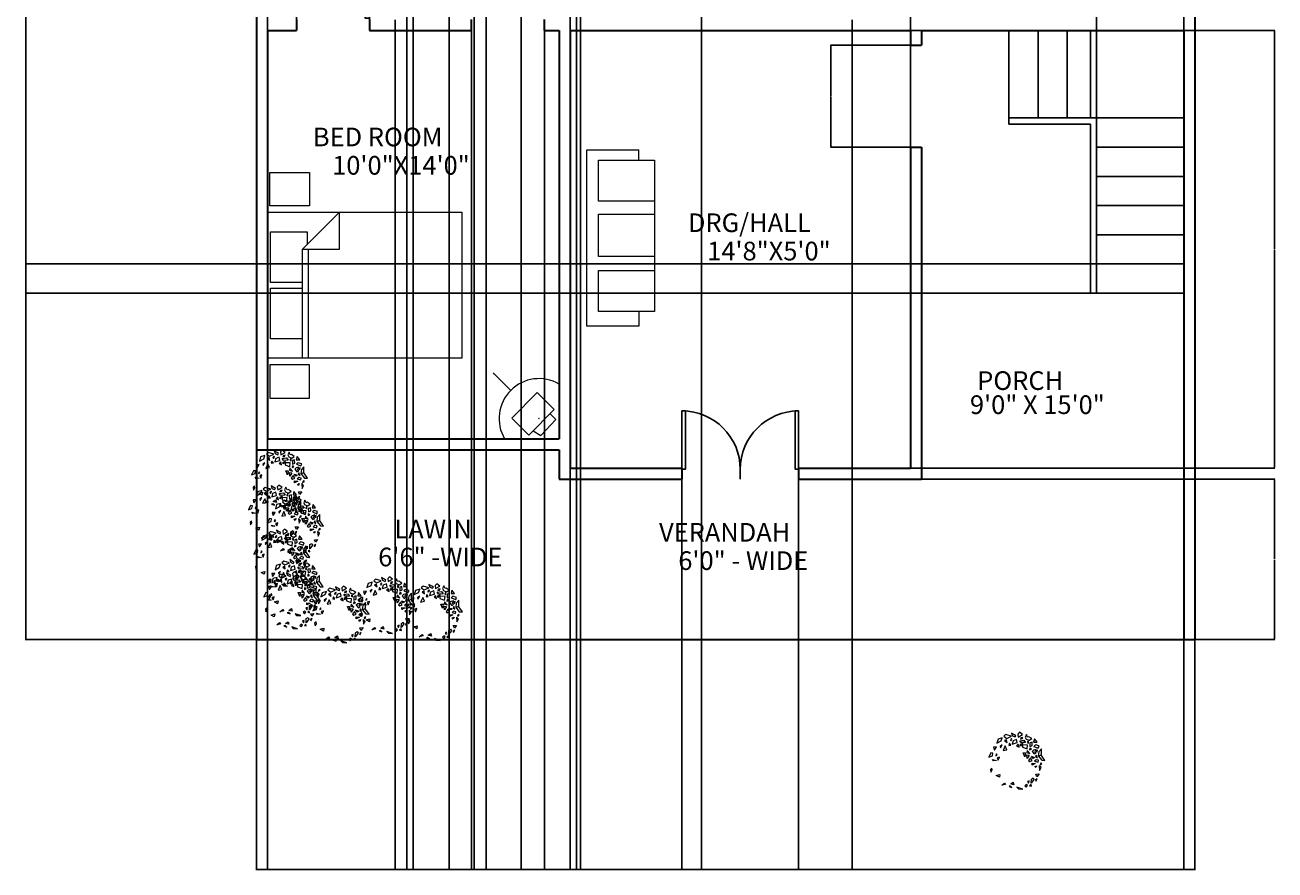
# Model space of a CAD drawing. Units: inches. Extents: x 2337 to 2851, y 1463 to 2183.
# Tile 1 of 4: x 2337 to 2851, y 1463 to 1810. Entities that reach past the tile are written whole.
import ezdxf

# ---------------------------------------------------------------- set-up
doc = ezdxf.new("R2010")
doc.units = ezdxf.units.IN
for name, color, linetype, lineweight in [('A-ANNO-DIMS', 2, 'Continuous', 18), ('A-AREA-IDEN', 7, 'Continuous', 18), ('A-DOOR', 4, 'Continuous', 25), ('A-FLOR-STRS', 7, 'Continuous', 25), ('A-FURN', 8, 'Continuous', 18), ('A-WALL', 7, 'Continuous', 35), ('L-PLNT-TREE', 94, 'Continuous', 13)]:
    doc.layers.add(name, color=color, linetype=linetype, lineweight=lineweight)
doc.styles.get("Standard").update_dxf_attribs({"font": 'arial.ttf'})
doc.dimstyles.get("Standard").update_dxf_attribs({"dimtxt": 0.18, "dimasz": 0.18, "dimexe": 0.18, "dimexo": 0.0625, "dimgap": 0.09, "dimtad": 0, "dimtih": 1, "dimtoh": 1, "dimdec": 4, "dimzin": 0, "dimdsep": 46, "dimtxsty": 'Standard', "dimcen": 0.09, "dimadec": 0, "dimazin": 0, "dimtfac": 1, "dimtdec": 4, "dimtofl": 0, "dimtmove": 0, "dimatfit": 3, "dimfxl": 1, "dimtolj": 1, "dimtzin": 0, "dimarcsym": 0})

# ---------------------------------------------------------------- blocks, each defined once
blk = doc.blocks.new('*U2')
for p, q in [((0, 0), (0, -5)), ((30, 0), (30, -5))]:
    blk.add_line(p, q)
blk.add_lwpolyline([(0, 0), (0, 30), (1.75, 30), (1.75, 0)], close=True)
blk.add_arc((0, 0), 30, 0, 90)
blk = doc.blocks.new('Bed - Queen')
for p, q in [((0, -80.00003), (0, 0)), ((0, 0), (59.99999, 0)), ((59.99999, 0), (59.99999, -80.00003)), ((7.99999, -1.2), (28.79998, -1.2)), ((7.99999, -14.4), (7.99999, -1.2)), ((28.79998, -1.2), (28.79998, -14.4)), ((31.19999, -1.2), (51.99999, -1.2)), ((31.19999, -14.4), (31.19999, -1.2)), ((51.99999, -1.2), (51.99999, -16.4)), ((0, -14.4), (44.8, -14.4)), ((59.99999, -29.6), (44.8, -14.4)), ((44.8, -14.4), (44.8, -29.6)), ((44.8, -16.8), (0, -16.8)), ((51.99999, -16.4), (46.79936, -16.4)), ((44.8, -29.6), (59.99999, -29.6)), ((59.99999, -80.00003), (0, -80.00003))]:
    blk.add_line(p, q)
blk = doc.blocks.new('*U10')
for points in [[(-4.43, 11.05), (-5.18, 10.36), (-3.96, 9.49), (-2.07, 10.36)], [(-2, 11.66), (-1.6, 10.62), (-0.52, 10.1), (-0.18, 10.62), (-0.79, 10.96)], [(1.24, 12), (0.56, 11.31), (0.76, 10.01), (2.52, 11.05)], [(4.14, 11.14), (3.6, 10.01), (4, 9.23), (5.22, 8.71), (6.3, 9.41), (5.08, 10.19), (4.61, 10.01)], [(-8.14, 6.03), (-9.36, 5.95), (-9.02, 4.73)], [(-5.78, 9.75), (-7.54, 9.23), (-8.01, 7.5), (-6.26, 8.45)], [(-5.78, 6.81), (-6.66, 6.21), (-6.52, 5.69)], [(-4.57, 6.38), (-5.45, 4.47), (-3.89, 4.82)], [(-4.84, 8.63), (-3.83, 7.85), (-4.03, 8.97)], [(-2.88, 7.5), (-3.15, 6.64), (-2.27, 6.72)], [(-1.94, 9.49), (-2.48, 8.97), (-2.27, 8.54), (-1.8, 9.06)], [(0.02, 9.06), (-1.33, 8.54), (-1.73, 7.16), (0.29, 7.76)], [(0.76, 7.16), (0.09, 6.46), (1.1, 5.95)], [(1.37, 8.54), (3.13, 8.8), (3.8, 7.85), (1.91, 7.76)], [(2.59, 9.93), (1.84, 9.75), (1.64, 9.23), (2.32, 9.41)], [(1.71, 6.29), (1.71, 7.07), (2.65, 7.5), (2.11, 6.9)], [(2.52, 6.81), (2.52, 5.86), (4.41, 5.17), (4.61, 6.72)], [(4.61, 8.28), (4.54, 7.76), (4.95, 7.59), (4.95, 8.28)], [(5.49, 5.51), (5.42, 4.82), (6.16, 5.08)], [(6.43, 7.94), (5.49, 7.68), (5.56, 6.21), (6.5, 6.64)], [(7.45, 9.32), (7.11, 7.94), (8.52, 7.94)], [(7.85, 6.81), (7.18, 6.21), (9, 5.51), (9.33, 6.38)], [(10.28, 5.17), (9.2, 4.04), (9, 2.31), (10.48, 0.49), (11.76, 0.41), (10.35, 2.48), (9.33, 2.4), (10.28, 2.83)], [(-11.32, 1.79), (-9.83, 2.31), (-9.63, 3.44), (-10.44, 3.52)], [(-8.21, 0.41), (-9.43, 0.32), (-9.83, 0.84)], [(-8.21, 3.09), (-8.48, 2.31), (-7.87, 2.57)], [(-7, 1.79), (-7.94, 1.53), (-7.47, 0.49)], [(3.53, 1.88), (2.86, 3.52), (3.8, 3.52)], [(4.41, 4.56), (4.27, 3.7), (5.49, 3.26)], [(4.27, 2.74), (5.29, 2.66), (4.41, 1.27)], [(5.83, 1.53), (5.02, 0.41), (5.49, -0.02), (6.5, 0.41)], [(7.51, 1.71), (6.91, 1.27), (6.23, 2.14)], [(8.12, 4.99), (7.11, 4.65), (6.5, 4.13), (7.38, 3.09), (8.12, 3.52), (7.65, 3.87)], [(8.12, 0.75), (7.51, 0.15), (8.93, -0.28), (9.13, 0.49)], [(8.19, 2.57), (7.92, 2.05), (8.66, 1.53)], [(8.73, 4.73), (8.19, 4.56), (8.39, 3.87), (8.59, 4.04)], [(-10.03, -2.71), (-10.64, -3.31), (-10.44, -4.44), (-9.9, -3.49)], [(7.78, -0.8), (6.43, -1.5), (6.43, -0.72)], [(8.32, -1.75), (7.98, -2.53), (7.58, -2.1)], [(9.33, -5.13), (8.46, -6.25), (7.98, -5.22)], [(9.33, -1.75), (9.54, -3.74), (10.14, -2.53)], [(10.08, -0.63), (9.74, -1.32), (10.48, -0.89)], [(-8.28, -5.73), (-6.79, -5.3), (-7, -6.51)], [(-4.84, -8.85), (-4.43, -9.45), (-5.99, -9.8)], [(-2.54, -10.06), (-3.02, -10.23), (-1.8, -10.67)], [(-2.34, -9.2), (-1.26, -8.5), (-0.99, -9.54)], [(4.07, -9.45), (3.53, -9.97), (4.07, -10.58), (4.61, -9.89)], [(5.29, -7.98), (4.61, -8.16), (5.02, -8.94)], [(6.03, -9.45), (5.42, -9.97), (6.16, -10.15)], [(6.1, -8.94), (6.16, -7.21), (6.91, -6.69), (7.24, -7.38)], [(8.05, -8.07), (8.59, -7.12), (7.92, -7.55)], [(0.22, -10.58), (0.83, -11.27), (2.59, -11.36)]]:
    blk.add_lwpolyline(points, close=True)
blk = doc.blocks.new('NIGHTSTAND')
blk.add_lwpolyline([(0, 13.73), (16.32, 13.73), (16.32, 0), (0, 0)], close=True)
blk = doc.blocks.new('*D29')
at = {"layer": 'A-ANNO-DIMS', "color": 0, "lineweight": -2, "transparency": 16777216}
for p, q in [((2432.04, 1557.27), (2432.04, 1462.52)), ((2818.04, 1557.27), (2818.04, 1462.52)), ((2432.22, 1462.7), (2624.75, 1462.7)), ((2817.86, 1462.7), (2625.33, 1462.7))]:
    blk.add_line(p, q, dxfattribs=at)
at = {"layer": 'A-ANNO-DIMS', "color": 0, "transparency": 16777216}
for points in [[(2432.22, 1462.73), (2432.22, 1462.67), (2432.04, 1462.7)], [(2817.86, 1462.73), (2817.86, 1462.67), (2818.04, 1462.7)]]:
    blk.add_solid(points, dxfattribs=at)
at = {"layer": 'Defpoints', "color": 0, "transparency": 16777216}
for p in [(2432.04, 1557.33), (2818.04, 1557.33), (2818.04, 1462.7)]:
    blk.add_point(p, dxfattribs=at)
at = {"layer": 'A-ANNO-DIMS', "color": 0, "transparency": 16777216, "insert": (2625.04, 1462.7), "char_height": 0.18, "attachment_point": 5}
blk.add_mtext('\\A1;386', dxfattribs=at)
blk = doc.blocks.new('*D30')
at = {"layer": 'A-ANNO-DIMS', "color": 0, "lineweight": -2, "transparency": 16777216}
for p, q in [((2431.97, 2149.83), (2336.95, 2149.83)), ((2337.13, 2149.65), (2337.13, 1853.76)), ((2337.13, 1557.51), (2337.13, 1853.4)), ((2431.97, 1557.33), (2336.95, 1557.33))]:
    blk.add_line(p, q, dxfattribs=at)
at = {"layer": 'A-ANNO-DIMS', "color": 0, "transparency": 16777216}
for points in [[(2337.1, 2149.65), (2337.16, 2149.65), (2337.13, 2149.83)], [(2337.1, 1557.51), (2337.16, 1557.51), (2337.13, 1557.33)]]:
    blk.add_solid(points, dxfattribs=at)
at = {"layer": 'Defpoints', "color": 0, "transparency": 16777216}
for p in [(2337.13, 2149.83), (2432.04, 2149.83), (2432.04, 1557.33)]:
    blk.add_point(p, dxfattribs=at)
at = {"layer": 'A-ANNO-DIMS', "color": 0, "transparency": 16777216, "insert": (2337.13, 1853.58), "char_height": 0.18, "attachment_point": 5}
blk.add_mtext('\\A1;592.5', dxfattribs=at)
blk = doc.blocks.new('*D32')
at = {"layer": 'A-ANNO-DIMS', "color": 0, "lineweight": -2, "transparency": 16777216}
for p, q in [((2561.04, 1627.89), (2561.04, 2182.75)), ((2561.22, 2182.57), (2630.76, 2182.57)), ((2700.86, 2182.57), (2631.32, 2182.57)), ((2701.04, 1627.89), (2701.04, 2182.75))]:
    blk.add_line(p, q, dxfattribs=at)
at = {"layer": 'A-ANNO-DIMS', "color": 0, "transparency": 16777216}
for points in [[(2561.22, 2182.6), (2561.22, 2182.54), (2561.04, 2182.57)], [(2700.86, 2182.6), (2700.86, 2182.54), (2701.04, 2182.57)]]:
    blk.add_solid(points, dxfattribs=at)
at = {"layer": 'Defpoints', "color": 0, "transparency": 16777216}
for p in [(2701.04, 2182.57), (2561.04, 1627.83), (2701.04, 1627.83)]:
    blk.add_point(p, dxfattribs=at)
at = {"layer": 'A-ANNO-DIMS', "color": 0, "transparency": 16777216, "insert": (2631.04, 2182.57), "char_height": 0.18, "attachment_point": 5}
blk.add_mtext('\\A1;140', dxfattribs=at)
blk = doc.blocks.new('*D33')
at = {"layer": 'A-ANNO-DIMS', "color": 0, "lineweight": -2, "transparency": 16777216}
for p, q in [((2701.1, 1807.83), (2850.96, 1807.83)), ((2850.78, 1807.65), (2850.78, 1718.01)), ((2850.78, 1628.01), (2850.78, 1717.65)), ((2701.1, 1627.83), (2850.96, 1627.83))]:
    blk.add_line(p, q, dxfattribs=at)
at = {"layer": 'A-ANNO-DIMS', "color": 0, "transparency": 16777216}
for points in [[(2850.75, 1807.65), (2850.81, 1807.65), (2850.78, 1807.83)], [(2850.75, 1628.01), (2850.81, 1628.01), (2850.78, 1627.83)]]:
    blk.add_solid(points, dxfattribs=at)
at = {"layer": 'Defpoints', "color": 0, "transparency": 16777216}
for p in [(2701.04, 1807.83), (2850.78, 1807.83), (2701.04, 1627.83)]:
    blk.add_point(p, dxfattribs=at)
at = {"layer": 'A-ANNO-DIMS', "color": 0, "transparency": 16777216, "insert": (2850.78, 1717.83), "char_height": 0.18, "attachment_point": 5}
blk.add_mtext('\\A1;180', dxfattribs=at)
blk = doc.blocks.new('*D35')
at = {"layer": 'A-ANNO-DIMS', "color": 0, "lineweight": -2, "transparency": 16777216}
for p, q in [((2489.04, 1812.27), (2489.04, 1462.52)), ((2677.04, 1812.27), (2677.04, 1462.52)), ((2489.22, 1462.7), (2582.76, 1462.7)), ((2676.86, 1462.7), (2583.32, 1462.7))]:
    blk.add_line(p, q, dxfattribs=at)
at = {"layer": 'A-ANNO-DIMS', "color": 0, "transparency": 16777216}
for points in [[(2489.22, 1462.73), (2489.22, 1462.67), (2489.04, 1462.7)], [(2676.86, 1462.73), (2676.86, 1462.67), (2677.04, 1462.7)]]:
    blk.add_solid(points, dxfattribs=at)
at = {"layer": 'Defpoints', "color": 0, "transparency": 16777216}
for p in [(2489.04, 1812.33), (2677.04, 1812.33), (2677.04, 1462.7)]:
    blk.add_point(p, dxfattribs=at)
at = {"layer": 'A-ANNO-DIMS', "color": 0, "transparency": 16777216, "insert": (2583.04, 1462.7), "char_height": 0.18, "attachment_point": 5}
blk.add_mtext('\\A1;188', dxfattribs=at)
blk = doc.blocks.new('*D37')
at = {"layer": 'A-ANNO-DIMS', "color": 0, "lineweight": -2, "transparency": 16777216}
for p, q in [((2615.04, 2080.77), (2615.04, 1462.52)), ((2813.54, 2080.77), (2813.54, 1462.52)), ((2615.22, 1462.7), (2713.9, 1462.7)), ((2813.36, 1462.7), (2714.67, 1462.7))]:
    blk.add_line(p, q, dxfattribs=at)
at = {"layer": 'A-ANNO-DIMS', "color": 0, "transparency": 16777216}
for points in [[(2615.22, 1462.73), (2615.22, 1462.67), (2615.04, 1462.7)], [(2813.36, 1462.73), (2813.36, 1462.67), (2813.54, 1462.7)]]:
    blk.add_solid(points, dxfattribs=at)
at = {"layer": 'Defpoints', "color": 0, "transparency": 16777216}
for p in [(2615.04, 2080.83), (2813.54, 2080.83), (2813.54, 1462.7)]:
    blk.add_point(p, dxfattribs=at)
at = {"layer": 'A-ANNO-DIMS', "color": 0, "transparency": 16777216, "insert": (2714.29, 1462.7), "char_height": 0.18, "attachment_point": 5}
blk.add_mtext('\\A1;198.5', dxfattribs=at)
blk = doc.blocks.new('*D38')
at = {"layer": 'A-ANNO-DIMS', "color": 0, "lineweight": -2, "transparency": 16777216}
for p, q in [((2496.54, 2080.77), (2496.54, 1462.52)), ((2526.54, 2080.77), (2526.54, 1462.52)), ((2496.72, 1462.7), (2511.32, 1462.7)), ((2526.36, 1462.7), (2511.76, 1462.7))]:
    blk.add_line(p, q, dxfattribs=at)
at = {"layer": 'A-ANNO-DIMS', "color": 0, "transparency": 16777216}
for points in [[(2496.72, 1462.73), (2496.72, 1462.67), (2496.54, 1462.7)], [(2526.36, 1462.73), (2526.36, 1462.67), (2526.54, 1462.7)]]:
    blk.add_solid(points, dxfattribs=at)
at = {"layer": 'Defpoints', "color": 0, "transparency": 16777216}
for p in [(2496.54, 2080.83), (2526.54, 2080.83), (2526.54, 1462.7)]:
    blk.add_point(p, dxfattribs=at)
at = {"layer": 'A-ANNO-DIMS', "color": 0, "transparency": 16777216, "insert": (2511.54, 1462.7), "char_height": 0.18, "attachment_point": 5}
blk.add_mtext('\\A1;30', dxfattribs=at)
blk = doc.blocks.new('*D39')
at = {"layer": 'A-ANNO-DIMS', "color": 0, "lineweight": -2, "transparency": 16777216}
for p, q in [((2607.04, 1623.27), (2607.04, 1462.52)), ((2655.04, 1623.27), (2655.04, 1462.52)), ((2607.22, 1462.7), (2630.81, 1462.7)), ((2654.86, 1462.7), (2631.26, 1462.7))]:
    blk.add_line(p, q, dxfattribs=at)
at = {"layer": 'A-ANNO-DIMS', "color": 0, "transparency": 16777216}
for points in [[(2607.22, 1462.73), (2607.22, 1462.67), (2607.04, 1462.7)], [(2654.86, 1462.73), (2654.86, 1462.67), (2655.04, 1462.7)]]:
    blk.add_solid(points, dxfattribs=at)
at = {"layer": 'Defpoints', "color": 0, "transparency": 16777216}
for p in [(2607.04, 1623.33), (2655.04, 1623.33), (2655.04, 1462.7)]:
    blk.add_point(p, dxfattribs=at)
at = {"layer": 'A-ANNO-DIMS', "color": 0, "transparency": 16777216, "insert": (2631.04, 1462.7), "char_height": 0.18, "attachment_point": 5}
blk.add_mtext('\\A1;48', dxfattribs=at)
blk = doc.blocks.new('*D43')
at = {"layer": 'A-ANNO-DIMS', "color": 0, "lineweight": -2, "transparency": 16777216}
for p, q in [((2520.54, 1807.77), (2520.54, 1462.52)), ((2550.54, 1807.77), (2550.54, 1462.52)), ((2520.72, 1462.7), (2535.32, 1462.7)), ((2550.36, 1462.7), (2535.76, 1462.7))]:
    blk.add_line(p, q, dxfattribs=at)
at = {"layer": 'A-ANNO-DIMS', "color": 0, "transparency": 16777216}
for points in [[(2520.72, 1462.73), (2520.72, 1462.67), (2520.54, 1462.7)], [(2550.36, 1462.73), (2550.36, 1462.67), (2550.54, 1462.7)]]:
    blk.add_solid(points, dxfattribs=at)
at = {"layer": 'Defpoints', "color": 0, "transparency": 16777216}
for p in [(2520.54, 1807.83), (2550.54, 1807.83), (2550.54, 1462.7)]:
    blk.add_point(p, dxfattribs=at)
at = {"layer": 'A-ANNO-DIMS', "color": 0, "transparency": 16777216, "insert": (2535.54, 1462.7), "char_height": 0.18, "attachment_point": 5}
blk.add_mtext('\\A1;30', dxfattribs=at)
blk = doc.blocks.new('*D44')
at = {"layer": 'A-ANNO-DIMS', "color": 0, "lineweight": -2, "transparency": 16777216}
for p, q in [((2436.54, 2085.27), (2436.54, 1462.52)), ((2496.54, 2085.27), (2496.54, 1462.52)), ((2436.72, 1462.7), (2466.32, 1462.7)), ((2496.36, 1462.7), (2466.76, 1462.7))]:
    blk.add_line(p, q, dxfattribs=at)
at = {"layer": 'A-ANNO-DIMS', "color": 0, "transparency": 16777216}
for points in [[(2436.72, 1462.73), (2436.72, 1462.67), (2436.54, 1462.7)], [(2496.36, 1462.73), (2496.36, 1462.67), (2496.54, 1462.7)]]:
    blk.add_solid(points, dxfattribs=at)
at = {"layer": 'Defpoints', "color": 0, "transparency": 16777216}
for p in [(2436.54, 2085.33), (2496.54, 2085.33), (2496.54, 1462.7)]:
    blk.add_point(p, dxfattribs=at)
at = {"layer": 'A-ANNO-DIMS', "color": 0, "transparency": 16777216, "insert": (2466.54, 1462.7), "char_height": 0.18, "attachment_point": 5}
blk.add_mtext('\\A1;60', dxfattribs=at)
blk = doc.blocks.new('*D45')
at = {"layer": 'A-ANNO-DIMS', "color": 0, "lineweight": -2, "transparency": 16777216}
for p, q in [((2777.54, 1699.89), (2777.54, 2182.75)), ((2777.72, 2182.57), (2795.32, 2182.57)), ((2813.36, 2182.57), (2795.76, 2182.57)), ((2813.54, 1699.89), (2813.54, 2182.75))]:
    blk.add_line(p, q, dxfattribs=at)
at = {"layer": 'A-ANNO-DIMS', "color": 0, "transparency": 16777216}
for points in [[(2777.72, 2182.6), (2777.72, 2182.54), (2777.54, 2182.57)], [(2813.36, 2182.6), (2813.36, 2182.54), (2813.54, 2182.57)]]:
    blk.add_solid(points, dxfattribs=at)
at = {"layer": 'Defpoints', "color": 0, "transparency": 16777216}
for p in [(2813.54, 2182.57), (2777.54, 1699.83), (2813.54, 1699.83)]:
    blk.add_point(p, dxfattribs=at)
at = {"layer": 'A-ANNO-DIMS', "color": 0, "transparency": 16777216, "insert": (2795.54, 2182.57), "char_height": 0.18, "attachment_point": 5}
blk.add_mtext('\\A1;36', dxfattribs=at)
blk = doc.blocks.new('*D46')
at = {"layer": 'A-ANNO-DIMS', "color": 0, "lineweight": -2, "transparency": 16777216}
for p, q in [((2777.47, 1711.83), (2336.95, 1711.83)), ((2337.13, 1711.65), (2337.13, 1706.01)), ((2337.13, 1700.01), (2337.13, 1705.65)), ((2777.47, 1699.83), (2336.95, 1699.83))]:
    blk.add_line(p, q, dxfattribs=at)
at = {"layer": 'A-ANNO-DIMS', "color": 0, "transparency": 16777216}
for points in [[(2337.1, 1711.65), (2337.16, 1711.65), (2337.13, 1711.83)], [(2337.1, 1700.01), (2337.16, 1700.01), (2337.13, 1699.83)]]:
    blk.add_solid(points, dxfattribs=at)
at = {"layer": 'Defpoints', "color": 0, "transparency": 16777216}
for p in [(2337.13, 1711.83), (2777.54, 1711.83), (2777.54, 1699.83)]:
    blk.add_point(p, dxfattribs=at)
at = {"layer": 'A-ANNO-DIMS', "color": 0, "transparency": 16777216, "insert": (2337.13, 1705.83), "char_height": 0.18, "attachment_point": 5}
blk.add_mtext('\\A1;12', dxfattribs=at)
blk = doc.blocks.new('*D50')
at = {"layer": 'A-ANNO-DIMS', "color": 0, "lineweight": -2, "transparency": 16777216}
for p, q in [((2493.91, 1831.57), (2493.91, 1462.52)), ((2521.63, 1831.57), (2521.63, 1462.52)), ((2494.09, 1462.7), (2507.3, 1462.7)), ((2521.45, 1462.7), (2508.23, 1462.7))]:
    blk.add_line(p, q, dxfattribs=at)
at = {"layer": 'A-ANNO-DIMS', "color": 0, "transparency": 16777216}
for points in [[(2494.09, 1462.73), (2494.09, 1462.67), (2493.91, 1462.7)], [(2521.45, 1462.73), (2521.45, 1462.67), (2521.63, 1462.7)]]:
    blk.add_solid(points, dxfattribs=at)
at = {"layer": 'Defpoints', "color": 0, "transparency": 16777216}
for p in [(2493.91, 1831.63), (2521.63, 1831.63), (2521.63, 1462.7)]:
    blk.add_point(p, dxfattribs=at)
at = {"layer": 'A-ANNO-DIMS', "color": 0, "transparency": 16777216, "insert": (2507.77, 1462.7), "char_height": 0.18, "attachment_point": 5}
blk.add_mtext('\\A1;27.724', dxfattribs=at)
blk = doc.blocks.new('*D51')
at = {"layer": 'A-ANNO-DIMS', "color": 0, "lineweight": -2, "transparency": 16777216}
for p, q in [((2511.27, 1939.17), (2511.27, 1462.52)), ((2563.65, 1939.17), (2563.65, 1462.52)), ((2511.45, 1462.7), (2537.06, 1462.7)), ((2563.47, 1462.7), (2537.85, 1462.7))]:
    blk.add_line(p, q, dxfattribs=at)
at = {"layer": 'A-ANNO-DIMS', "color": 0, "transparency": 16777216}
for points in [[(2511.45, 1462.73), (2511.45, 1462.67), (2511.27, 1462.7)], [(2563.47, 1462.73), (2563.47, 1462.67), (2563.65, 1462.7)]]:
    blk.add_solid(points, dxfattribs=at)
at = {"layer": 'Defpoints', "color": 0, "transparency": 16777216}
for p in [(2511.27, 1939.23), (2563.65, 1939.23), (2563.65, 1462.7)]:
    blk.add_point(p, dxfattribs=at)
at = {"layer": 'A-ANNO-DIMS', "color": 0, "transparency": 16777216, "insert": (2537.46, 1462.7), "char_height": 0.18, "attachment_point": 5}
blk.add_mtext('\\A1;52.38', dxfattribs=at)
blk = doc.blocks.new('*D53')
at = {"layer": 'A-ANNO-DIMS', "color": 0, "lineweight": -2, "transparency": 16777216}
for p, q in [((2540.84, 1848.69), (2540.84, 1462.52)), ((2565.31, 1848.69), (2565.31, 1462.52)), ((2541.02, 1462.7), (2552.61, 1462.7)), ((2565.13, 1462.7), (2553.54, 1462.7))]:
    blk.add_line(p, q, dxfattribs=at)
at = {"layer": 'A-ANNO-DIMS', "color": 0, "transparency": 16777216}
for points in [[(2541.02, 1462.73), (2541.02, 1462.67), (2540.84, 1462.7)], [(2565.13, 1462.73), (2565.13, 1462.67), (2565.31, 1462.7)]]:
    blk.add_solid(points, dxfattribs=at)
at = {"layer": 'Defpoints', "color": 0, "transparency": 16777216}
for p in [(2540.84, 1848.75), (2565.31, 1848.75), (2565.31, 1462.7)]:
    blk.add_point(p, dxfattribs=at)
at = {"layer": 'A-ANNO-DIMS', "color": 0, "transparency": 16777216, "insert": (2553.08, 1462.7), "char_height": 0.18, "attachment_point": 5}
blk.add_mtext('\\A1;24.466', dxfattribs=at)
blk = doc.blocks.new('*D55')
at = {"layer": 'A-ANNO-DIMS', "color": 0, "lineweight": -2, "transparency": 16777216}
for p, q in [((2705.6, 1623.33), (2850.96, 1623.33)), ((2850.78, 1623.15), (2850.78, 1590.51)), ((2850.78, 1557.51), (2850.78, 1590.15)), ((2813.6, 1557.33), (2850.96, 1557.33))]:
    blk.add_line(p, q, dxfattribs=at)
at = {"layer": 'A-ANNO-DIMS', "color": 0, "transparency": 16777216}
for points in [[(2850.75, 1623.15), (2850.81, 1623.15), (2850.78, 1623.33)], [(2850.75, 1557.51), (2850.81, 1557.51), (2850.78, 1557.33)]]:
    blk.add_solid(points, dxfattribs=at)
at = {"layer": 'Defpoints', "color": 0, "transparency": 16777216}
for p in [(2705.54, 1623.33), (2813.54, 1557.33), (2850.78, 1557.33)]:
    blk.add_point(p, dxfattribs=at)
at = {"layer": 'A-ANNO-DIMS', "color": 0, "transparency": 16777216, "insert": (2850.78, 1590.33), "char_height": 0.18, "attachment_point": 5}
blk.add_mtext('\\A1;66', dxfattribs=at)
blk = doc.blocks.new('*D56')
at = {"layer": 'A-ANNO-DIMS', "color": 0, "lineweight": -2, "transparency": 16777216}
for p, q in [((2700.97, 1801.83), (2668.12, 1801.83)), ((2668.3, 1801.65), (2668.3, 1781.01)), ((2668.3, 1760.01), (2668.3, 1780.65)), ((2700.97, 1759.83), (2668.12, 1759.83))]:
    blk.add_line(p, q, dxfattribs=at)
at = {"layer": 'A-ANNO-DIMS', "color": 0, "transparency": 16777216}
for points in [[(2668.27, 1801.65), (2668.33, 1801.65), (2668.3, 1801.83)], [(2668.27, 1760.01), (2668.33, 1760.01), (2668.3, 1759.83)]]:
    blk.add_solid(points, dxfattribs=at)
at = {"layer": 'Defpoints', "color": 0, "transparency": 16777216}
for p in [(2668.3, 1801.83), (2701.04, 1801.83), (2701.04, 1759.83)]:
    blk.add_point(p, dxfattribs=at)
at = {"layer": 'A-ANNO-DIMS', "color": 0, "transparency": 16777216, "insert": (2668.3, 1780.83), "char_height": 0.18, "attachment_point": 5}
blk.add_mtext('\\A1;42', dxfattribs=at)
blk = doc.blocks.new('*D59')
at = {"layer": 'A-ANNO-DIMS', "color": 0, "lineweight": -2, "transparency": 16777216}
for p, q in [((2561.04, 1627.77), (2561.04, 1462.52)), ((2607.04, 1627.77), (2607.04, 1462.52)), ((2561.22, 1462.7), (2583.81, 1462.7)), ((2606.86, 1462.7), (2584.26, 1462.7))]:
    blk.add_line(p, q, dxfattribs=at)
at = {"layer": 'A-ANNO-DIMS', "color": 0, "transparency": 16777216}
for points in [[(2561.22, 1462.73), (2561.22, 1462.67), (2561.04, 1462.7)], [(2606.86, 1462.73), (2606.86, 1462.67), (2607.04, 1462.7)]]:
    blk.add_solid(points, dxfattribs=at)
at = {"layer": 'Defpoints', "color": 0, "transparency": 16777216}
for p in [(2561.04, 1627.83), (2607.04, 1627.83), (2607.04, 1462.7)]:
    blk.add_point(p, dxfattribs=at)
at = {"layer": 'A-ANNO-DIMS', "color": 0, "transparency": 16777216, "insert": (2584.04, 1462.7), "char_height": 0.18, "attachment_point": 5}
blk.add_mtext('\\A1;46', dxfattribs=at)
blk = doc.blocks.new('*D61')
at = {"layer": 'A-ANNO-DIMS', "color": 0, "lineweight": -2, "transparency": 16777216}
for p, q in [((2529.43, 1666.73), (2529.61, 1666.73)), ((2529.61, 1666.73), (2536.47, 1659.91)), ((2548.15, 1648.2), (2548.33, 1648.2)), ((2548.24, 1648.11), (2548.24, 1648.29))]:
    blk.add_line(p, q, dxfattribs=at)
at = {"layer": 'A-ANNO-DIMS', "color": 0, "transparency": 16777216}
blk.add_solid([(2536.49, 1659.93), (2536.45, 1659.89), (2536.59, 1659.78)], dxfattribs=at)
at = {"layer": 'Defpoints', "color": 0, "transparency": 16777216}
for p in [(2536.59, 1659.78), (2548.24, 1648.2)]:
    blk.add_point(p, dxfattribs=at)
at = {"layer": 'A-ANNO-DIMS', "color": 0, "transparency": 16777216, "insert": (2528.88, 1666.73), "char_height": 0.18, "attachment_point": 5}
blk.add_mtext('\\A1;R16.423', dxfattribs=at)

msp = doc.modelspace()

# ---------------------------------------------------------------- linework, layer by layer
at = {"layer": 'A-FLOR-STRS'}
for p, q in [((2741.5375, 1807.828), (2741.5375, 1769.328)), ((2753.5375, 1807.828), (2753.5375, 1771.828)), ((2765.5375, 1807.828), (2765.5375, 1771.828)), ((2775.0375, 1807.828), (2775.0375, 1771.828)), ((2741.5375, 1771.828), (2813.5375, 1771.828)), ((2741.5375, 1769.328), (2775.0375, 1769.328)), ((2741.5375, 1769.328), (2775.0375, 1769.328)), ((2775.0375, 1769.328), (2775.0375, 1699.828)), ((2777.5375, 1771.828), (2777.5375, 1699.828)), ((2777.5375, 1759.828), (2813.5375, 1759.828)), ((2777.5375, 1747.828), (2813.5375, 1747.828)), ((2777.5375, 1735.828), (2813.5375, 1735.828)), ((2777.5375, 1723.828), (2813.5375, 1723.828)), ((2777.5375, 1711.828), (2813.5375, 1711.828)), ((2775.0375, 1699.828), (2813.5375, 1699.828))]:
    msp.add_line(p, q, dxfattribs=at)
at = {"layer": 'A-FURN'}
for p, q in [((2589.3112, 1754.4706), (2589.3112, 1758.6721)), ((2589.3112, 1692.2664), (2589.3112, 1686.2155)), ((2548.9544, 1641.226), (2555.1419, 1647.8474)), ((2555.1419, 1647.8474), (2552.7922, 1650.1652)), ((2545.8967, 1643.175), (2548.9544, 1641.226))]:
    msp.add_line(p, q, dxfattribs=at)
for points in [[(2589.3112, 1686.2155), (2567.963, 1686.2155), (2567.963, 1758.6721), (2589.3112, 1758.6721)], [(2595.6869, 1754.4706), (2595.6869, 1692.2664)]]:
    msp.add_lwpolyline(points, dxfattribs=at)
for points in [[(2572.7379, 1754.4706), (2595.6869, 1754.4706), (2595.6869, 1737.558), (2572.7379, 1737.558)], [(2572.7379, 1732.2387), (2595.6869, 1732.2387), (2595.6869, 1714.9081), (2572.7379, 1714.9081)], [(2572.7379, 1709.038), (2595.6869, 1709.038), (2595.6869, 1692.2664), (2572.7379, 1692.2664)], [(2537.0803, 1648.313), (2547.5057, 1658.8818), (2554.5429, 1651.94), (2544.1175, 1641.3712)]]:
    msp.add_lwpolyline(points, close=True, dxfattribs=at)
msp.add_arc((2548.2366, 1648.2022), 16.4228, 59.639116, 210.658134, dxfattribs=at)
at = {"layer": 'A-WALL'}
for p, q in [((2432.0375, 2149.828), (2432.0375, 1557.328)), ((2818.0375, 2149.828), (2818.0375, 1557.328)), ((2448.5375, 1812.328), (2448.5375, 1807.828)), ((2478.5375, 1812.328), (2478.5375, 1807.828)), ((2520.5375, 1807.828), (2520.5375, 1812.328)), ((2550.5375, 1807.828), (2550.5375, 1812.328)), ((2436.5375, 1807.828), (2448.5375, 1807.828)), ((2436.5375, 1807.828), (2436.5375, 1639.828)), ((2478.5375, 1807.828), (2520.5375, 1807.828)), ((2550.5375, 1807.828), (2556.5375, 1807.828)), ((2556.5375, 1807.828), (2556.5375, 1639.828)), ((2561.0375, 1807.828), (2561.0375, 1627.828)), ((2561.0375, 1807.828), (2701.0375, 1807.828)), ((2701.0375, 1807.828), (2701.0375, 1801.828)), ((2705.5375, 1807.828), (2705.5375, 1801.828)), ((2705.5375, 1807.828), (2813.5375, 1807.828)), ((2813.5375, 1807.828), (2813.5375, 1557.328)), ((2701.0375, 1801.828), (2705.5375, 1801.828)), ((2701.0375, 1759.828), (2705.5375, 1759.828)), ((2701.0375, 1759.828), (2701.0375, 1627.828)), ((2705.5375, 1759.828), (2705.5375, 1623.328)), ((2432.0375, 1635.328), (2556.5375, 1635.328)), ((2436.5375, 1639.828), (2556.5375, 1639.828)), ((2556.5375, 1635.328), (2556.5375, 1623.328)), ((2561.0375, 1627.828), (2607.0375, 1627.828)), ((2607.0375, 1627.828), (2607.0375, 1623.328)), ((2655.0375, 1627.828), (2655.0375, 1623.328)), ((2655.0375, 1627.828), (2701.0375, 1627.828)), ((2556.5375, 1623.328), (2607.0375, 1623.328)), ((2655.0375, 1623.328), (2705.5375, 1623.328)), ((2432.0375, 1557.328), (2818.0375, 1557.328))]:
    msp.add_line(p, q, dxfattribs=at)

# ---------------------------------------------------------------- block references
at = {"layer": 'A-DOOR', "xscale": -1}
msp.add_blockref('*U2', (2478.5375, 1812.828), dxfattribs=at)
at = {"layer": 'A-DOOR', "yscale": 0.8, "zscale": 0.8}
for p, xscale in [((2607.0375, 1627.328), 0.8), ((2655.0375, 1627.328), -0.8)]:
    msp.add_blockref('*U2', p, dxfattribs=dict(at, xscale=xscale))
at = {"layer": 'A-FURN'}
msp.add_blockref('NIGHTSTAND', (2437.506, 1735.705), dxfattribs=at)
at = {"layer": 'A-FURN', "rotation": 90}
msp.add_blockref('Bed - Queen', (2436.5375, 1673.0338), dxfattribs=at)
at = {"layer": 'A-FURN', "extrusion": (0, 0, -1), "zscale": -1, "rotation": 180}
msp.add_blockref('NIGHTSTAND', (-2437.506, 1670.3626), dxfattribs=at)
at = {"layer": 'L-PLNT-TREE'}
for p in [(2441.2931, 1623.244), (2440.0135, 1608.8663), (2447.8526, 1603.5649), (2442.2528, 1590.6545), (2447.6911, 1578.5133), (2446.3522, 1573.1259), (2466.5651, 1567.3306), (2485.4597, 1571.1514), (2504.9735, 1568.2759), (2744.6002, 1507.1491)]:
    msp.add_blockref('*U10', p, dxfattribs=at)

# ---------------------------------------------------------------- texts
at = {"layer": 'A-AREA-IDEN'}
for s, height, p in [('BED ROOM', 7.67227, (2455.2497, 1760.1791)), ('10\'0"X14\'0"', 7.672274, (2463.1779, 1748.5274)), ('DRG/HALL', 7.67227, (2609.5102, 1724.9117)), ('14\'8"X5\'0"', 7.67227, (2617.4384, 1713.26)), ('PORCH', 7.67227, (2728.5005, 1659.9736)), ('9\'0" X 15\'0"', 7.672274, (2725.5039, 1650.0754)), ('LAWIN', 7.67227, (2488.7734, 1598.8774)), ('VERANDAH', 7.67227, (2597.6233, 1597.5863)), ('6\'6" -WIDE', 7.67227, (2482.1104, 1587.42)), ('6\'0" - WIDE', 7.672274, (2605.5515, 1585.9346))]:
    msp.add_text(s, height=height, dxfattribs=at).set_placement(p)

# ---------------------------------------------------------------- dimensions: what is measured, and where the dimension line sits
at = {"layer": 'A-ANNO-DIMS'}
for base, p1, p2, override, picture, middle in [((2701.0375, 2182.568), (2561.0375, 1627.828), (2701.0375, 1627.828), {"dimdec": 0, "dimlfac": 1, "dimrnd": 0, "dimzin": 0, "dimdsep": 46, "dimlunit": 2}, '*D32', (2631.0375, 2182.568)), ((2813.5375, 2182.568), (2777.5375, 1699.828), (2813.5375, 1699.828), {"dimdec": 0, "dimlfac": 1, "dimrnd": 0, "dimzin": 0, "dimdsep": 46, "dimlunit": 2}, '*D45', (2795.5375, 2182.568)), ((2496.5375, 1462.7036), (2436.5375, 2085.328), (2496.5375, 2085.328), {"dimdec": 0, "dimlfac": 1, "dimrnd": 0, "dimzin": 0, "dimdsep": 46, "dimlunit": 2}, '*D44', (2466.5375, 1462.7036)), ((2526.5375, 1462.7036), (2496.5375, 2080.828), (2526.5375, 2080.828), {"dimdec": 0, "dimlfac": 1, "dimrnd": 0, "dimzin": 0, "dimdsep": 46, "dimlunit": 2}, '*D38', (2511.5375, 1462.7036)), ((2813.5375, 1462.7036), (2615.0375, 2080.828), (2813.5375, 2080.828), {"dimdec": 1, "dimlfac": 1, "dimrnd": 0, "dimzin": 0, "dimdsep": 46, "dimlunit": 2}, '*D37', (2714.2875, 1462.7036)), ((2563.646, 1462.7036), (2511.2705, 1939.2296), (2563.646, 1939.2296), {"dimdec": 2, "dimlfac": 1, "dimrnd": 0, "dimzin": 0, "dimdsep": 46, "dimlunit": 2}, '*D51', (2537.4582, 1462.7036)), ((2565.3084, 1462.7036), (2540.8421, 1848.7517), (2565.3084, 1848.7517), {"dimdec": 3, "dimlfac": 1, "dimrnd": 0, "dimzin": 0, "dimdsep": 46, "dimlunit": 2}, '*D53', (2553.0753, 1462.7036)), ((2521.6304, 1462.7036), (2493.9066, 1831.6316), (2521.6304, 1831.6316), {"dimdec": 3, "dimlfac": 1, "dimrnd": 0, "dimzin": 0, "dimdsep": 46, "dimlunit": 2}, '*D50', (2507.7685, 1462.7036)), ((2677.0375, 1462.7036), (2489.0375, 1812.328), (2677.0375, 1812.328), {"dimdec": 0, "dimlfac": 1, "dimrnd": 0, "dimzin": 0, "dimdsep": 46, "dimlunit": 2}, '*D35', (2583.0375, 1462.7036)), ((2550.5375, 1462.7036), (2520.5375, 1807.828), (2550.5375, 1807.828), {"dimdec": 0, "dimlfac": 1, "dimrnd": 0, "dimzin": 0, "dimdsep": 46, "dimlunit": 2}, '*D43', (2535.5375, 1462.7036)), ((2607.0375, 1462.7036), (2561.0375, 1627.828), (2607.0375, 1627.828), {"dimdec": 0, "dimlfac": 1, "dimrnd": 0, "dimzin": 0, "dimdsep": 46, "dimlunit": 2}, '*D59', (2584.0375, 1462.7036)), ((2655.0375, 1462.7036), (2607.0375, 1623.328), (2655.0375, 1623.328), {"dimdec": 0, "dimlfac": 1, "dimrnd": 0, "dimzin": 0, "dimdsep": 46, "dimlunit": 2}, '*D39', (2631.0375, 1462.7036)), ((2818.0375, 1462.7036), (2432.0375, 1557.328), (2818.0375, 1557.328), {"dimdec": 0, "dimlfac": 1, "dimrnd": 0, "dimzin": 0, "dimdsep": 46, "dimlunit": 2}, '*D29', (2625.0375, 1462.7036))]:
    dim = msp.add_linear_dim(base=base, p1=p1, p2=p2, dimstyle='Standard', override=override, dxfattribs=at)
    dim.commit()
    dim.dimension.update_dxf_attribs({"geometry": picture, "text_midpoint": middle})
for base, p1, p2, override, picture, middle in [((2337.1275, 2149.828), (2432.0375, 1557.328), (2432.0375, 2149.828), {"dimdec": 1, "dimlfac": 1, "dimrnd": 0, "dimzin": 0, "dimdsep": 46, "dimlunit": 2}, '*D30', (2337.1275, 1853.578)), ((2850.7775, 1807.828), (2701.0375, 1627.828), (2701.0375, 1807.828), {"dimdec": 0, "dimlfac": 1, "dimrnd": 0, "dimzin": 0, "dimdsep": 46, "dimlunit": 2}, '*D33', (2850.7775, 1717.828)), ((2668.2975, 1801.828), (2701.0375, 1759.828), (2701.0375, 1801.828), {"dimdec": 0, "dimlfac": 1, "dimrnd": 0, "dimzin": 0, "dimdsep": 46, "dimlunit": 2}, '*D56', (2668.2975, 1780.828)), ((2337.1275, 1711.828), (2777.5375, 1699.828), (2777.5375, 1711.828), {"dimdec": 0, "dimlfac": 1, "dimrnd": 0, "dimzin": 0, "dimdsep": 46, "dimlunit": 2}, '*D46', (2337.1275, 1705.828)), ((2850.7775, 1557.328), (2705.5375, 1623.328), (2813.5375, 1557.328), {"dimdec": 0, "dimlfac": 1, "dimrnd": 0, "dimzin": 0, "dimdsep": 46, "dimlunit": 2}, '*D55', (2850.7775, 1590.328))]:
    dim = msp.add_linear_dim(base=base, p1=p1, p2=p2, angle=90, dimstyle='Standard', override=override, dxfattribs=at)
    dim.commit()
    dim.dimension.update_dxf_attribs({"geometry": picture, "text_midpoint": middle})
dim = msp.add_radius_dim(center=(2548.2366, 1648.2022), mpoint=(2536.5941, 1659.7849), dimstyle='Standard', override={"dimdec": 3, "dimlfac": 1, "dimrnd": 0, "dimzin": 0, "dimdsep": 46, "dimlunit": 2}, dxfattribs=at)
dim.commit()
dim.dimension.update_dxf_attribs({"geometry": '*D61', "text_midpoint": (2528.8788, 1666.7345), "dimtype": 164})

doc.saveas('drawing.dxf')
